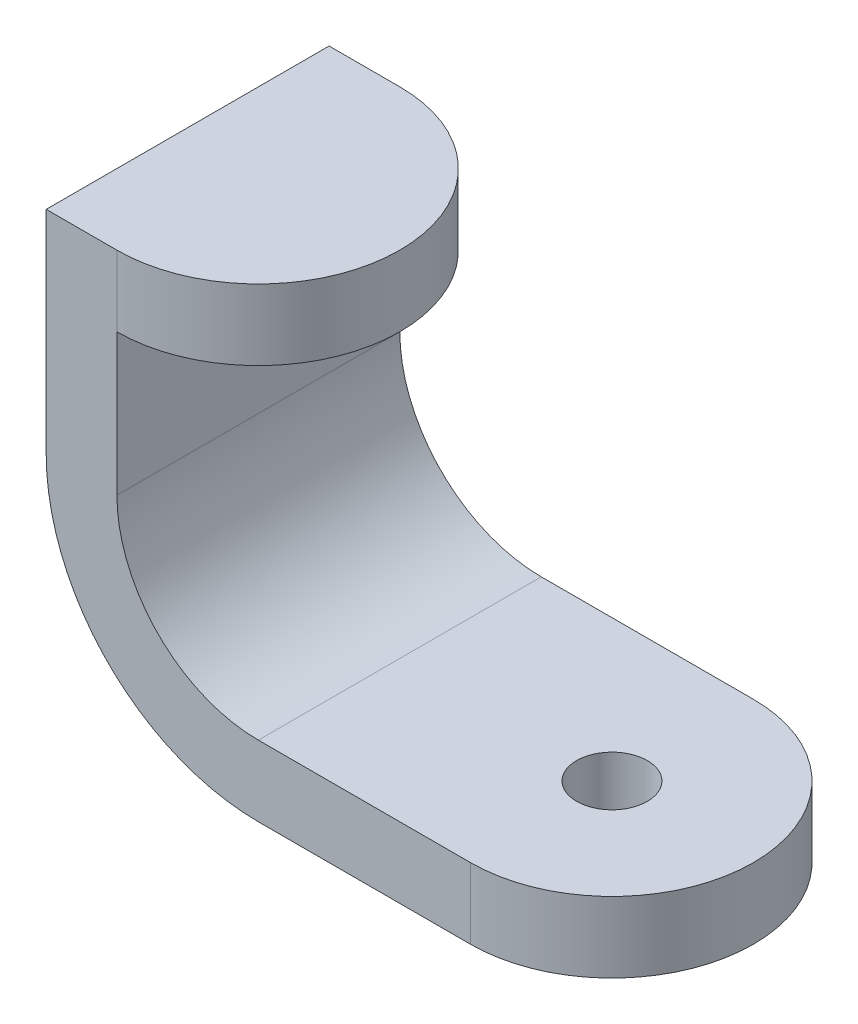
ISO-10303-21;
HEADER;
FILE_DESCRIPTION(('STEP AP214'),'2;1');
FILE_NAME('part.step','',(''),(''),'','','');
FILE_SCHEMA(('AUTOMOTIVE_DESIGN { 1 0 10303 214 1 1 1 1 }'));
ENDSEC;
DATA;
#1=APPLICATION_CONTEXT('core data for automotive mechanical design processes');
#2=APPLICATION_PROTOCOL_DEFINITION('international standard','automotive_design',2000,#1);
#3=PRODUCT_CONTEXT('',#1,'mechanical');
#4=PRODUCT('Part','Part','',(#3));
#5=PRODUCT_RELATED_PRODUCT_CATEGORY('part','',(#4));
#6=PRODUCT_DEFINITION_FORMATION('','',#4);
#7=PRODUCT_DEFINITION_CONTEXT('part definition',#1,'design');
#8=PRODUCT_DEFINITION('design','',#6,#7);
#9=PRODUCT_DEFINITION_SHAPE('','',#8);
#10=(LENGTH_UNIT() NAMED_UNIT(*) SI_UNIT(.MILLI.,.METRE.));
#11=(NAMED_UNIT(*) PLANE_ANGLE_UNIT() SI_UNIT($,.RADIAN.));
#12=(NAMED_UNIT(*) SI_UNIT($,.STERADIAN.) SOLID_ANGLE_UNIT());
#13=UNCERTAINTY_MEASURE_WITH_UNIT(LENGTH_MEASURE(1.E-05),#10,'distance_accuracy_value','');
#14=(GEOMETRIC_REPRESENTATION_CONTEXT(3) GLOBAL_UNCERTAINTY_ASSIGNED_CONTEXT((#13)) GLOBAL_UNIT_ASSIGNED_CONTEXT((#10,
#11,#12)) REPRESENTATION_CONTEXT('',''));
#15=CARTESIAN_POINT('',(0.,0.,0.));
#16=DIRECTION('',(0.,0.,1.));
#17=DIRECTION('',(1.,0.,0.));
#18=AXIS2_PLACEMENT_3D('',#15,#16,#17);
#19=CARTESIAN_POINT('',(0.,20.0000000000001,40.));
#20=DIRECTION('',(1.,0.,0.));
#21=DIRECTION('',(0.,0.,-1.));
#22=AXIS2_PLACEMENT_3D('',#19,#20,#21);
#23=PLANE('',#22);
#24=DIRECTION('',(0.,-1.,0.));
#25=VECTOR('',#24,1.);
#26=CARTESIAN_POINT('',(0.,20.0000000000001,0.));
#27=LINE('',#26,#25);
#28=CARTESIAN_POINT('',(0.,40.,0.));
#29=VERTEX_POINT('',#28);
#30=CARTESIAN_POINT('',(0.,20.0000000000001,0.));
#31=VERTEX_POINT('',#30);
#32=EDGE_CURVE('E155',#29,#31,#27,.T.);
#33=ORIENTED_EDGE('',*,*,#32,.F.);
#34=DIRECTION('',(0.,0.,1.));
#35=VECTOR('',#34,1.);
#36=CARTESIAN_POINT('',(0.,40.,0.));
#37=LINE('',#36,#35);
#38=CARTESIAN_POINT('',(0.,40.,40.));
#39=VERTEX_POINT('',#38);
#40=EDGE_CURVE('E56',#29,#39,#37,.T.);
#41=ORIENTED_EDGE('',*,*,#40,.T.);
#42=DIRECTION('',(0.,-1.,0.));
#43=VECTOR('',#42,1.);
#44=CARTESIAN_POINT('',(0.,20.0000000000001,40.));
#45=LINE('',#44,#43);
#46=CARTESIAN_POINT('',(0.,20.0000000000001,40.));
#47=VERTEX_POINT('',#46);
#48=EDGE_CURVE('E135',#39,#47,#45,.T.);
#49=ORIENTED_EDGE('',*,*,#48,.T.);
#50=DIRECTION('',(0.,0.,-1.));
#51=VECTOR('',#50,1.);
#52=CARTESIAN_POINT('',(0.,20.0000000000001,40.));
#53=LINE('',#52,#51);
#54=EDGE_CURVE('E52',#47,#31,#53,.T.);
#55=ORIENTED_EDGE('',*,*,#54,.T.);
#56=EDGE_LOOP('',(#33,#41,#49,#55));
#57=FACE_BOUND('',#56,.T.);
#58=ADVANCED_FACE('F44',(#57),#23,.T.);
#59=CARTESIAN_POINT('',(20.0000000000001,-10.,40.));
#60=DIRECTION('',(0.,1.,0.));
#61=DIRECTION('',(0.,0.,1.));
#62=AXIS2_PLACEMENT_3D('',#59,#60,#61);
#63=PLANE('',#62);
#64=CARTESIAN_POINT('',(50.,-10.,20.));
#65=DIRECTION('',(0.,1.,0.));
#66=DIRECTION('',(0.,0.,1.));
#67=AXIS2_PLACEMENT_3D('',#64,#65,#66);
#68=CIRCLE('',#67,5.);
#69=CARTESIAN_POINT('',(50.,-10.,25.));
#70=VERTEX_POINT('',#69);
#71=EDGE_CURVE('E239',#70,#70,#68,.T.);
#72=ORIENTED_EDGE('',*,*,#71,.T.);
#73=EDGE_LOOP('',(#72));
#74=FACE_BOUND('',#73,.T.);
#75=DIRECTION('',(1.,0.,0.));
#76=VECTOR('',#75,1.);
#77=CARTESIAN_POINT('',(20.0000000000001,-10.,0.));
#78=LINE('',#77,#76);
#79=CARTESIAN_POINT('',(20.0000000000001,-10.,0.));
#80=VERTEX_POINT('',#79);
#81=CARTESIAN_POINT('',(50.,-10.,0.));
#82=VERTEX_POINT('',#81);
#83=EDGE_CURVE('E138',#80,#82,#78,.T.);
#84=ORIENTED_EDGE('',*,*,#83,.T.);
#85=CARTESIAN_POINT('',(50.,-10.,20.));
#86=DIRECTION('',(0.,1.,0.));
#87=DIRECTION('',(0.,0.,1.));
#88=AXIS2_PLACEMENT_3D('',#85,#86,#87);
#89=CIRCLE('',#88,20.);
#90=CARTESIAN_POINT('',(50.,-10.,40.));
#91=VERTEX_POINT('',#90);
#92=EDGE_CURVE('E181',#91,#82,#89,.T.);
#93=ORIENTED_EDGE('',*,*,#92,.F.);
#94=DIRECTION('',(1.,0.,0.));
#95=VECTOR('',#94,1.);
#96=CARTESIAN_POINT('',(20.0000000000001,-10.,40.));
#97=LINE('',#96,#95);
#98=CARTESIAN_POINT('',(20.0000000000001,-10.,40.));
#99=VERTEX_POINT('',#98);
#100=EDGE_CURVE('E159',#99,#91,#97,.T.);
#101=ORIENTED_EDGE('',*,*,#100,.F.);
#102=DIRECTION('',(0.,0.,-1.));
#103=VECTOR('',#102,1.);
#104=CARTESIAN_POINT('',(20.0000000000001,-10.,40.));
#105=LINE('',#104,#103);
#106=EDGE_CURVE('E136',#99,#80,#105,.T.);
#107=ORIENTED_EDGE('',*,*,#106,.T.);
#108=EDGE_LOOP('',(#84,#93,#101,#107));
#109=FACE_BOUND('',#108,.T.);
#110=ADVANCED_FACE('F50',(#74,#109),#63,.F.);
#111=CARTESIAN_POINT('',(20.0000000000001,0.,40.));
#112=DIRECTION('',(0.,1.,0.));
#113=DIRECTION('',(0.,0.,1.));
#114=AXIS2_PLACEMENT_3D('',#111,#112,#113);
#115=PLANE('',#114);
#116=CARTESIAN_POINT('',(50.,0.,20.));
#117=DIRECTION('',(0.,1.,0.));
#118=DIRECTION('',(0.,0.,1.));
#119=AXIS2_PLACEMENT_3D('',#116,#117,#118);
#120=CIRCLE('',#119,5.);
#121=CARTESIAN_POINT('',(50.,0.,25.));
#122=VERTEX_POINT('',#121);
#123=EDGE_CURVE('E240',#122,#122,#120,.T.);
#124=ORIENTED_EDGE('',*,*,#123,.F.);
#125=EDGE_LOOP('',(#124));
#126=FACE_BOUND('',#125,.T.);
#127=DIRECTION('',(1.,0.,0.));
#128=VECTOR('',#127,1.);
#129=CARTESIAN_POINT('',(20.0000000000001,0.,0.));
#130=LINE('',#129,#128);
#131=CARTESIAN_POINT('',(20.0000000000001,0.,0.));
#132=VERTEX_POINT('',#131);
#133=CARTESIAN_POINT('',(50.,0.,0.));
#134=VERTEX_POINT('',#133);
#135=EDGE_CURVE('E148',#132,#134,#130,.T.);
#136=ORIENTED_EDGE('',*,*,#135,.F.);
#137=DIRECTION('',(0.,0.,-1.));
#138=VECTOR('',#137,1.);
#139=CARTESIAN_POINT('',(20.0000000000001,0.,40.));
#140=LINE('',#139,#138);
#141=CARTESIAN_POINT('',(20.0000000000001,0.,40.));
#142=VERTEX_POINT('',#141);
#143=EDGE_CURVE('E11',#142,#132,#140,.T.);
#144=ORIENTED_EDGE('',*,*,#143,.F.);
#145=DIRECTION('',(1.,0.,0.));
#146=VECTOR('',#145,1.);
#147=CARTESIAN_POINT('',(20.0000000000001,0.,40.));
#148=LINE('',#147,#146);
#149=CARTESIAN_POINT('',(50.,0.,40.));
#150=VERTEX_POINT('',#149);
#151=EDGE_CURVE('E191',#142,#150,#148,.T.);
#152=ORIENTED_EDGE('',*,*,#151,.T.);
#153=CARTESIAN_POINT('',(50.,0.,20.));
#154=DIRECTION('',(0.,1.,0.));
#155=DIRECTION('',(0.,0.,1.));
#156=AXIS2_PLACEMENT_3D('',#153,#154,#155);
#157=CIRCLE('',#156,20.);
#158=EDGE_CURVE('E188',#150,#134,#157,.T.);
#159=ORIENTED_EDGE('',*,*,#158,.T.);
#160=EDGE_LOOP('',(#136,#144,#152,#159));
#161=FACE_BOUND('',#160,.T.);
#162=ADVANCED_FACE('F200',(#126,#161),#115,.T.);
#163=CARTESIAN_POINT('',(20.,20.,40.));
#164=DIRECTION('',(0.,0.,-1.));
#165=DIRECTION('',(-1.,0.,0.));
#166=AXIS2_PLACEMENT_3D('',#163,#164,#165);
#167=CYLINDRICAL_SURFACE('',#166,20.);
#168=CARTESIAN_POINT('',(20.,20.,0.));
#169=DIRECTION('',(0.,0.,1.));
#170=DIRECTION('',(-1.,0.,0.));
#171=AXIS2_PLACEMENT_3D('',#168,#169,#170);
#172=CIRCLE('',#171,20.);
#173=EDGE_CURVE('E149',#31,#132,#172,.T.);
#174=ORIENTED_EDGE('',*,*,#173,.F.);
#175=ORIENTED_EDGE('',*,*,#54,.F.);
#176=CARTESIAN_POINT('',(20.,20.,40.));
#177=DIRECTION('',(0.,0.,1.));
#178=DIRECTION('',(-1.,0.,0.));
#179=AXIS2_PLACEMENT_3D('',#176,#177,#178);
#180=CIRCLE('',#179,20.);
#181=EDGE_CURVE('E193',#47,#142,#180,.T.);
#182=ORIENTED_EDGE('',*,*,#181,.T.);
#183=ORIENTED_EDGE('',*,*,#143,.T.);
#184=EDGE_LOOP('',(#174,#175,#182,#183));
#185=FACE_BOUND('',#184,.T.);
#186=ADVANCED_FACE('F168',(#185),#167,.F.);
#187=CARTESIAN_POINT('',(-10.,50.,40.));
#188=DIRECTION('',(0.,1.,0.));
#189=DIRECTION('',(0.,0.,1.));
#190=AXIS2_PLACEMENT_3D('',#187,#188,#189);
#191=PLANE('',#190);
#192=DIRECTION('',(1.,0.,0.));
#193=VECTOR('',#192,1.);
#194=CARTESIAN_POINT('',(-10.,50.,0.));
#195=LINE('',#194,#193);
#196=CARTESIAN_POINT('',(-10.,50.,0.));
#197=VERTEX_POINT('',#196);
#198=CARTESIAN_POINT('',(0.,50.,0.));
#199=VERTEX_POINT('',#198);
#200=EDGE_CURVE('E120',#197,#199,#195,.T.);
#201=ORIENTED_EDGE('',*,*,#200,.F.);
#202=DIRECTION('',(0.,0.,-1.));
#203=VECTOR('',#202,1.);
#204=CARTESIAN_POINT('',(-10.,50.,40.));
#205=LINE('',#204,#203);
#206=CARTESIAN_POINT('',(-10.,50.,40.));
#207=VERTEX_POINT('',#206);
#208=EDGE_CURVE('E115',#207,#197,#205,.T.);
#209=ORIENTED_EDGE('',*,*,#208,.F.);
#210=DIRECTION('',(1.,0.,0.));
#211=VECTOR('',#210,1.);
#212=CARTESIAN_POINT('',(-10.,50.,40.));
#213=LINE('',#212,#211);
#214=CARTESIAN_POINT('',(0.,50.,40.));
#215=VERTEX_POINT('',#214);
#216=EDGE_CURVE('E119',#207,#215,#213,.T.);
#217=ORIENTED_EDGE('',*,*,#216,.T.);
#218=CARTESIAN_POINT('',(0.,50.,20.));
#219=DIRECTION('',(0.,1.,0.));
#220=DIRECTION('',(0.,0.,1.));
#221=AXIS2_PLACEMENT_3D('',#218,#219,#220);
#222=CIRCLE('',#221,20.);
#223=EDGE_CURVE('E178',#215,#199,#222,.T.);
#224=ORIENTED_EDGE('',*,*,#223,.T.);
#225=EDGE_LOOP('',(#201,#209,#217,#224));
#226=FACE_BOUND('',#225,.T.);
#227=ADVANCED_FACE('F111',(#226),#191,.T.);
#228=CARTESIAN_POINT('',(-10.,20.0000000000001,40.));
#229=DIRECTION('',(1.,0.,0.));
#230=DIRECTION('',(0.,0.,-1.));
#231=AXIS2_PLACEMENT_3D('',#228,#229,#230);
#232=PLANE('',#231);
#233=DIRECTION('',(0.,1.,0.));
#234=VECTOR('',#233,1.);
#235=CARTESIAN_POINT('',(-10.,20.0000000000001,0.));
#236=LINE('',#235,#234);
#237=CARTESIAN_POINT('',(-10.,20.0000000000002,0.));
#238=VERTEX_POINT('',#237);
#239=EDGE_CURVE('E160',#197,#238,#236,.F.);
#240=ORIENTED_EDGE('',*,*,#239,.T.);
#241=DIRECTION('',(0.,0.,-1.));
#242=VECTOR('',#241,1.);
#243=CARTESIAN_POINT('',(-10.,20.0000000000002,40.));
#244=LINE('',#243,#242);
#245=CARTESIAN_POINT('',(-10.,20.0000000000002,40.));
#246=VERTEX_POINT('',#245);
#247=EDGE_CURVE('E125',#246,#238,#244,.T.);
#248=ORIENTED_EDGE('',*,*,#247,.F.);
#249=DIRECTION('',(0.,1.,0.));
#250=VECTOR('',#249,1.);
#251=CARTESIAN_POINT('',(-10.,20.0000000000001,40.));
#252=LINE('',#251,#250);
#253=EDGE_CURVE('E123',#207,#246,#252,.F.);
#254=ORIENTED_EDGE('',*,*,#253,.F.);
#255=ORIENTED_EDGE('',*,*,#208,.T.);
#256=EDGE_LOOP('',(#240,#248,#254,#255));
#257=FACE_BOUND('',#256,.T.);
#258=ADVANCED_FACE('F127',(#257),#232,.F.);
#259=CARTESIAN_POINT('',(20.,20.,40.));
#260=DIRECTION('',(0.,0.,-1.));
#261=DIRECTION('',(-1.,0.,0.));
#262=AXIS2_PLACEMENT_3D('',#259,#260,#261);
#263=CYLINDRICAL_SURFACE('',#262,30.);
#264=CARTESIAN_POINT('',(20.,20.,0.));
#265=DIRECTION('',(0.,0.,1.));
#266=DIRECTION('',(1.,0.,0.));
#267=AXIS2_PLACEMENT_3D('',#264,#265,#266);
#268=CIRCLE('',#267,30.);
#269=EDGE_CURVE('E94',#238,#80,#268,.T.);
#270=ORIENTED_EDGE('',*,*,#269,.T.);
#271=ORIENTED_EDGE('',*,*,#106,.F.);
#272=CARTESIAN_POINT('',(20.,20.,40.));
#273=DIRECTION('',(0.,0.,1.));
#274=DIRECTION('',(1.,0.,0.));
#275=AXIS2_PLACEMENT_3D('',#272,#273,#274);
#276=CIRCLE('',#275,30.);
#277=EDGE_CURVE('E69',#246,#99,#276,.T.);
#278=ORIENTED_EDGE('',*,*,#277,.F.);
#279=ORIENTED_EDGE('',*,*,#247,.T.);
#280=EDGE_LOOP('',(#270,#271,#278,#279));
#281=FACE_BOUND('',#280,.T.);
#282=ADVANCED_FACE('F269',(#281),#263,.T.);
#283=CARTESIAN_POINT('',(20.,20.,40.));
#284=DIRECTION('',(0.,0.,1.));
#285=DIRECTION('',(1.,0.,0.));
#286=AXIS2_PLACEMENT_3D('',#283,#284,#285);
#287=PLANE('',#286);
#288=ORIENTED_EDGE('',*,*,#100,.T.);
#289=DIRECTION('',(0.,-1.,0.));
#290=VECTOR('',#289,1.);
#291=CARTESIAN_POINT('',(50.,0.,40.));
#292=LINE('',#291,#290);
#293=EDGE_CURVE('E192',#150,#91,#292,.T.);
#294=ORIENTED_EDGE('',*,*,#293,.F.);
#295=ORIENTED_EDGE('',*,*,#151,.F.);
#296=ORIENTED_EDGE('',*,*,#181,.F.);
#297=ORIENTED_EDGE('',*,*,#48,.F.);
#298=EDGE_CURVE('E134',#215,#39,#45,.T.);
#299=ORIENTED_EDGE('',*,*,#298,.F.);
#300=ORIENTED_EDGE('',*,*,#216,.F.);
#301=ORIENTED_EDGE('',*,*,#253,.T.);
#302=ORIENTED_EDGE('',*,*,#277,.T.);
#303=EDGE_LOOP('',(#288,#294,#295,#296,#297,#299,#300,#301,#302));
#304=FACE_BOUND('',#303,.T.);
#305=ADVANCED_FACE('F129',(#304),#287,.T.);
#306=CARTESIAN_POINT('',(20.,20.,0.));
#307=DIRECTION('',(0.,0.,1.));
#308=DIRECTION('',(1.,0.,0.));
#309=AXIS2_PLACEMENT_3D('',#306,#307,#308);
#310=PLANE('',#309);
#311=ORIENTED_EDGE('',*,*,#83,.F.);
#312=ORIENTED_EDGE('',*,*,#269,.F.);
#313=ORIENTED_EDGE('',*,*,#239,.F.);
#314=ORIENTED_EDGE('',*,*,#200,.T.);
#315=EDGE_CURVE('E153',#199,#29,#27,.T.);
#316=ORIENTED_EDGE('',*,*,#315,.T.);
#317=ORIENTED_EDGE('',*,*,#32,.T.);
#318=ORIENTED_EDGE('',*,*,#173,.T.);
#319=ORIENTED_EDGE('',*,*,#135,.T.);
#320=DIRECTION('',(0.,-1.,0.));
#321=VECTOR('',#320,1.);
#322=CARTESIAN_POINT('',(50.,0.,0.));
#323=LINE('',#322,#321);
#324=EDGE_CURVE('E141',#134,#82,#323,.T.);
#325=ORIENTED_EDGE('',*,*,#324,.T.);
#326=EDGE_LOOP('',(#311,#312,#313,#314,#316,#317,#318,#319,#325));
#327=FACE_BOUND('',#326,.T.);
#328=ADVANCED_FACE('F172',(#327),#310,.F.);
#329=CARTESIAN_POINT('',(0.,40.,20.));
#330=DIRECTION('',(0.,1.,0.));
#331=DIRECTION('',(0.,0.,1.));
#332=AXIS2_PLACEMENT_3D('',#329,#330,#331);
#333=CYLINDRICAL_SURFACE('',#332,20.);
#334=ORIENTED_EDGE('',*,*,#223,.F.);
#335=ORIENTED_EDGE('',*,*,#298,.T.);
#336=CARTESIAN_POINT('',(0.,40.,20.));
#337=DIRECTION('',(0.,1.,0.));
#338=DIRECTION('',(0.,0.,1.));
#339=AXIS2_PLACEMENT_3D('',#336,#337,#338);
#340=CIRCLE('',#339,20.);
#341=EDGE_CURVE('E182',#39,#29,#340,.T.);
#342=ORIENTED_EDGE('',*,*,#341,.T.);
#343=ORIENTED_EDGE('',*,*,#315,.F.);
#344=EDGE_LOOP('',(#334,#335,#342,#343));
#345=FACE_BOUND('',#344,.T.);
#346=ADVANCED_FACE('F176',(#345),#333,.T.);
#347=CARTESIAN_POINT('',(0.,40.,20.));
#348=DIRECTION('',(0.,1.,0.));
#349=DIRECTION('',(0.,0.,1.));
#350=AXIS2_PLACEMENT_3D('',#347,#348,#349);
#351=PLANE('',#350);
#352=ORIENTED_EDGE('',*,*,#341,.F.);
#353=ORIENTED_EDGE('',*,*,#40,.F.);
#354=EDGE_LOOP('',(#352,#353));
#355=FACE_BOUND('',#354,.T.);
#356=ADVANCED_FACE('F210',(#355),#351,.F.);
#357=CARTESIAN_POINT('',(50.,-10.,20.));
#358=DIRECTION('',(0.,1.,0.));
#359=DIRECTION('',(0.,0.,1.));
#360=AXIS2_PLACEMENT_3D('',#357,#358,#359);
#361=CYLINDRICAL_SURFACE('',#360,20.);
#362=ORIENTED_EDGE('',*,*,#158,.F.);
#363=ORIENTED_EDGE('',*,*,#293,.T.);
#364=ORIENTED_EDGE('',*,*,#92,.T.);
#365=ORIENTED_EDGE('',*,*,#324,.F.);
#366=EDGE_LOOP('',(#362,#363,#364,#365));
#367=FACE_BOUND('',#366,.T.);
#368=ADVANCED_FACE('F207',(#367),#361,.T.);
#369=CARTESIAN_POINT('',(50.,-10.,20.));
#370=DIRECTION('',(0.,1.,0.));
#371=DIRECTION('',(0.,0.,1.));
#372=AXIS2_PLACEMENT_3D('',#369,#370,#371);
#373=CYLINDRICAL_SURFACE('',#372,5.);
#374=ORIENTED_EDGE('',*,*,#71,.F.);
#375=EDGE_LOOP('',(#374));
#376=FACE_BOUND('',#375,.T.);
#377=ORIENTED_EDGE('',*,*,#123,.T.);
#378=EDGE_LOOP('',(#377));
#379=FACE_BOUND('',#378,.T.);
#380=ADVANCED_FACE('F216',(#376,#379),#373,.F.);
#381=CLOSED_SHELL('',(#58,#110,#162,#186,#227,#258,#282,#305,#328,#346,#356,#368,#380));
#382=MANIFOLD_SOLID_BREP('B2',#381);
#383=ADVANCED_BREP_SHAPE_REPRESENTATION('',(#18,#382),#14);
#384=SHAPE_DEFINITION_REPRESENTATION(#9,#383);
ENDSEC;
END-ISO-10303-21;
